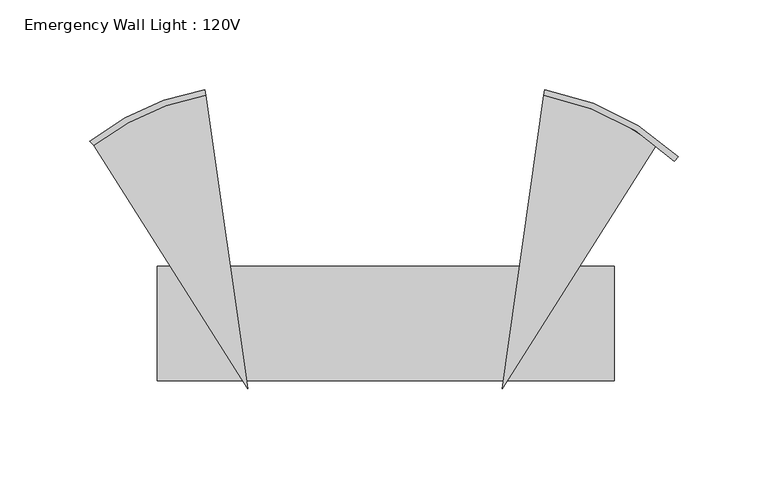
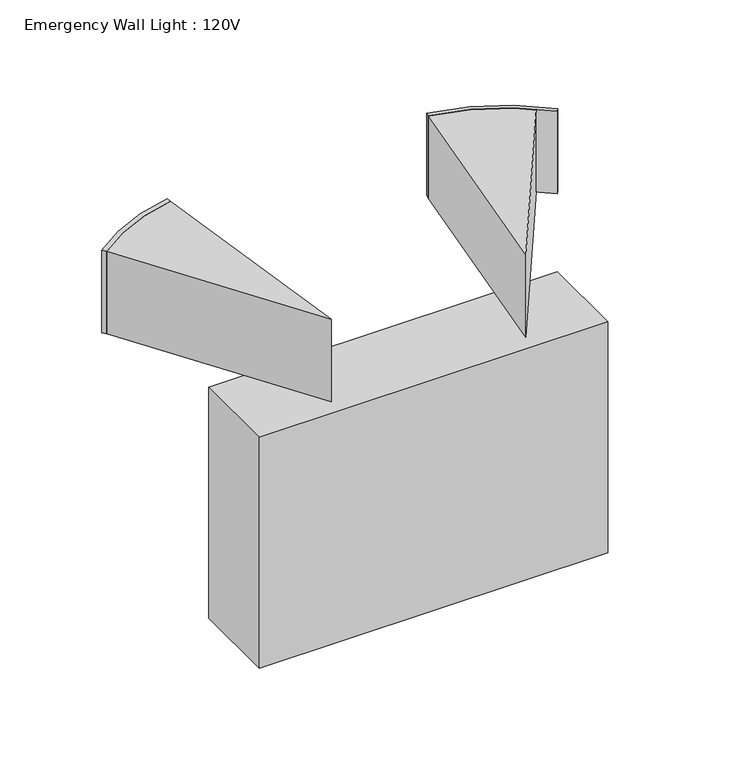
"""IFC4 building model written with IfcOpenShell, lengths in millimetres: light fixture geometry, Emergency Wall Light : 120V."""

from ifc_helpers import new_model, si_unit, point, frame, frame_2d, origin, place, context, project, spatial, polyline, circle_curve, trimmed, segment, composite_curve, outline, extrude, source, transform, mapped, element, save


def emergency_wall_light_120v_c8ddf26d(model_context):
    return source(origin(), model_context, "Body", "SweptSolid", [
        extrude(outline(polyline([(-127.0, 206.6635654), (127.0, 206.6635654), (127.0, 143.1635654), (-127.0, 143.1635654), (-127.0, 206.6635654)])), frame((0.0, 0.0, 2044.7), z_axis=(0.0, 0.0, 1.0), x_axis=(1.0, 0.0, 0.0)), (0.0, 0.0, 1.0), 177.8),
        extrude(outline(composite_curve([segment(polyline([(-162.5670168, 273.9397902), (-164.6100242, 276.3719813)]), True, "CONTINUOUS"), segment(trimmed(circle_curve(frame_2d((-76.8817714, 165.3727224)), 141.4817367), [point((-164.6100242, 276.3719813))], [point((-100.6159592, 304.8494951))], False, "CARTESIAN"), True, "CONTINUOUS"), segment(polyline([(-100.6159592, 304.8494951), (-100.0646262, 301.7227305)]), True, "CONTINUOUS"), segment(trimmed(circle_curve(frame_2d((-76.8817714, 165.3727224)), 138.3067948), [point((-100.0646262, 301.7227305))], [point((-162.5670168, 273.9397902))], True, "CARTESIAN"), True, "CONTINUOUS")], self_intersect=False)), frame((0.0, 0.0, 2235.2), z_axis=(0.0, 0.0, 1.0), x_axis=(1.0, 0.0, 0.0)), (0.0, 0.0, 1.0), 63.5),
        extrude(outline(composite_curve([segment(polyline([(87.8199065, 301.7227305), (88.3712395, 304.8494951)]), True, "CONTINUOUS"), segment(trimmed(circle_curve(frame_2d((64.6866749, 164.950378)), 141.8898219), [point((88.3712395, 304.8494951))], [point((162.6293819, 267.6146255))], False, "CARTESIAN"), True, "CONTINUOUS"), segment(polyline([(162.6293819, 267.6146255), (160.5885313, 265.1734131)]), True, "CONTINUOUS"), segment(trimmed(circle_curve(frame_2d((64.6866749, 164.950378)), 138.7148976), [point((160.5885313, 265.1734131))], [point((87.8199065, 301.7227305))], True, "CARTESIAN"), True, "CONTINUOUS")], self_intersect=False)), frame((0.0, 0.0, 2235.2), z_axis=(0.0, 0.0, 1.0), x_axis=(1.0, 0.0, 0.0)), (0.0, 0.0, 1.0), 63.5),
        extrude(outline(composite_curve([segment(polyline([(-100.0646262, 301.7227305), (-76.8817714, 138.5521459), (-162.5670168, 273.9397902)]), True, "CONTINUOUS"), segment(trimmed(circle_curve(frame_2d((-76.8817714, 165.3727224)), 138.3067948), [point((-162.5670168, 273.9397902))], [point((-100.0646262, 301.7227305))], False, "CARTESIAN"), True, "CONTINUOUS")], self_intersect=False)), frame((0.0, 0.0, 2235.2), z_axis=(0.0, 0.0, 1.0), x_axis=(1.0, 0.0, 0.0)), (0.0, 0.0, 1.0), 63.5),
        extrude(outline(composite_curve([segment(polyline([(64.6866749, 138.5521459), (87.8199065, 301.7227305)]), True, "CONTINUOUS"), segment(trimmed(circle_curve(frame_2d((64.6866749, 164.950378)), 138.7148976), [point((87.8199065, 301.7227305))], [point((150.4953624, 273.9397902))], False, "CARTESIAN"), True, "CONTINUOUS"), segment(polyline([(150.4953624, 273.9397902), (64.6866749, 138.5521459)]), True, "CONTINUOUS")], self_intersect=False)), frame((0.0, 0.0, 2235.2), z_axis=(0.0, 0.0, 1.0), x_axis=(1.0, 0.0, 0.0)), (0.0, 0.0, 1.0), 63.5),
    ])


if __name__ == "__main__":
    model = new_model("IFC4")
    model_context = context("Model", 3, world=origin())
    ifc_project = project(units=[si_unit("LENGTHUNIT", "METRE", prefix="MILLI")], contexts=[model_context])
    site = spatial("IfcSite", under=ifc_project)
    building = spatial("IfcBuilding", under=site)
    placement = place(None, origin())
    emergency_wall_light_120v_shape = emergency_wall_light_120v_c8ddf26d(model_context)
    element("IfcLightFixture", 1, ObjectType="Emergency Wall Light : 120V", at=placement, inside=building, context=model_context, shape_type="MappedRepresentation", body=[
        mapped(emergency_wall_light_120v_shape, transform((0.0, 0.0, 0.0), x_axis=(1.0, 0.0, 0.0), y_axis=(0.0, 1.0, 0.0), z_axis=(0.0, 0.0, 1.0))),
    ])
    save(model, "model.ifc")

# Revit data of these elements
# Type "Emergency Wall Light : 120V"
#   Lamp = "A-19"
#   Assembly Code = "D5090200"
#   Wattage Comments = "100"
#   Ballast Voltage = 120 V
#   Mounting Height = 7' - 0"
#   Apparent Load = 100 VA
#   Ballast Number of Poles = 1
#   Diffuser = Glass, White, High Luminance
#   Light Casing = Steel, Paint Finish, Ivory, Glossy
#   Default Elevation = 0
# Element 1 (IfcLightFixture, "Emergency Wall Light : 120V")
#   Materials on its faces: "Steel, Paint Finish, Ivory, Glossy", "Glass, White, High Luminance"
# Materials
#   "Glass, White, High Luminance": class "Glass", colour RGB 249 250 249, transparency 0.8, Description = "physical material", Cost = 0
#   "Steel, Paint Finish, Ivory, Glossy": class "Metal", colour RGB 247 247 239, transparency 0, Description = "Steel, paint finish, ivory, glossy", Cost = 0
